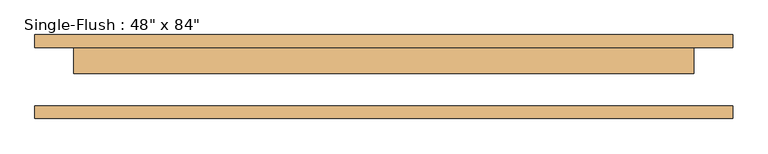
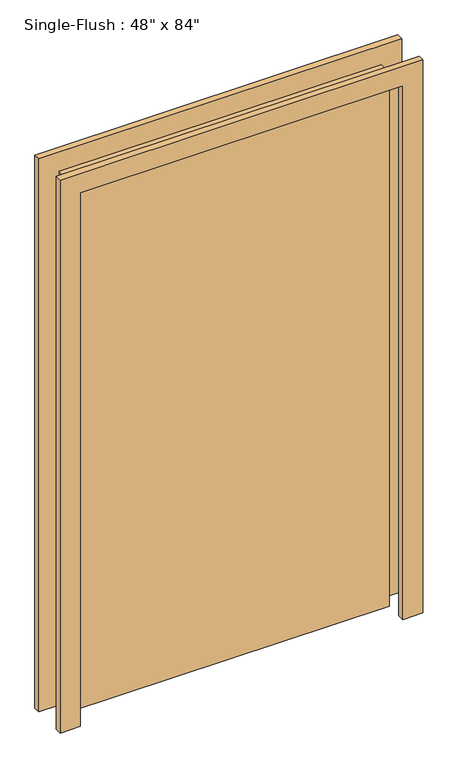
"""IFC4 building model written with IfcOpenShell, lengths in millimetres: door geometry."""

from ifc_helpers import new_model, si_unit, frame, origin, origin_with_axes, place, context, project, spatial, polyline, outline, extrude, source, transform, mapped, element, save


def door_6ea84ebe(model_context):
    return source(origin(), model_context, "Body", "SweptSolid", [
        extrude(outline(polyline([(2209.8, -685.8), (0.0, -685.8), (0.0, -609.6), (2133.6, -609.6), (2133.6, 609.6), (0.0, 609.6), (0.0, 685.8), (2209.8, 685.8), (2209.8, -685.8)])), frame((0.0, 57.15, 0.0), z_axis=(0.0, 1.0, 0.0), x_axis=(0.0, 0.0, 1.0)), (0.0, 0.0, 1.0), 25.4),
        extrude(outline(polyline([(2209.8, 685.8), (2209.8, -685.8), (0.0, -685.8), (0.0, -609.6), (2133.6, -609.6), (2133.6, 609.6), (0.0, 609.6), (0.0, 685.8), (2209.8, 685.8)])), frame((0.0, -82.55, 0.0), z_axis=(0.0, 1.0, 0.0), x_axis=(0.0, 0.0, 1.0)), (0.0, 0.0, 1.0), 25.4),
        extrude(outline(polyline([(609.6, 6.35), (-609.6, 6.35), (-609.6, 57.15), (609.6, 57.15), (609.6, 6.35)])), origin_with_axes(), (0.0, 0.0, 1.0), 2133.6),
    ])


if __name__ == "__main__":
    model = new_model("IFC4")
    model_context = context("Model", 3, world=origin())
    ifc_project = project(units=[si_unit("LENGTHUNIT", "METRE", prefix="MILLI")], contexts=[model_context])
    site = spatial("IfcSite", under=ifc_project)
    building = spatial("IfcBuilding", under=site)
    placement = place(None, origin())
    door_shape = door_6ea84ebe(model_context)
    element("IfcDoor", 1, ObjectType="Single-Flush : 48\" x 84\"", at=placement, inside=building, context=model_context, shape_type="MappedRepresentation", body=[
        mapped(door_shape, transform((0.0, 0.0, 0.0), x_axis=(1.0, 0.0, 0.0), y_axis=(0.0, 1.0, 0.0), z_axis=(0.0, 0.0, 1.0))),
    ])
    save(model, "model.ifc")

# Revit data of these elements
# Type "Single-Flush : 48\" x 84\""
#   Type Mark = "5"
#   Construction Type Id = "MDOOR"
#   Assembly Code = "C1020"
#   Analytic Construction = "Metal"
#   Thickness = 0' - 2"
#   Heat Transfer Coefficient (U) = 0.651978 BTU/(h·ft²·°F)
#   Height = 7' - 0"
#   Trim Projection Ext = 0' - 1"
#   Trim Projection Int = 0' - 1"
#   Trim Width = 0' - 3"
#   Width = 4' - 0"
#   Define Thermal Properties by = 1
#   Define Thermal Properties by = 1
#   Door Material = Door - Panel
#   Frame Material = Door - Frame
#   Visual Light Transmittance = 0
#   Solar Heat Gain Coefficient = 0
#   Function = (empty or 0)
#   Wall Closure = (empty or 0)
# Element 1 (IfcDoor, "Single-Flush : 48\" x 84\"")
#   Materials on its faces: "Door - Frame", "Door - Panel"
# Materials
#   "Door - Panel": class "Wood", colour RGB 210 159 95, transparency 0, Cost = 0
#   "Door - Frame": colour RGB 118 70 51, transparency 0, Cost = 0
